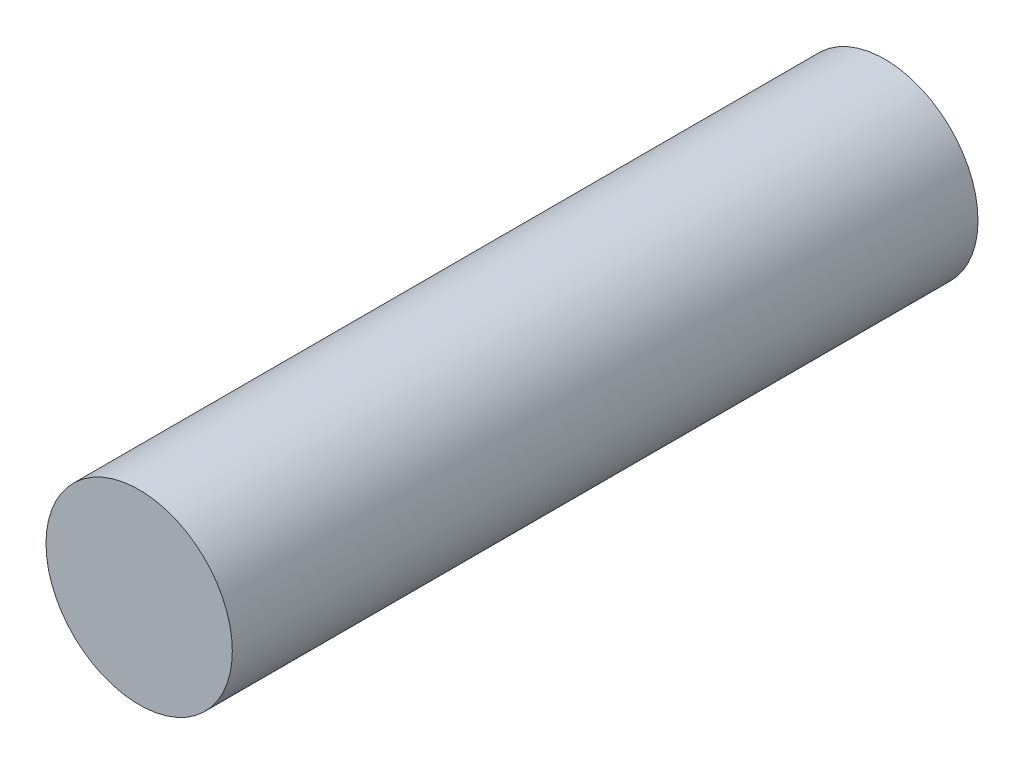
SolidWorks part; units mm, degrees
material "Plain Carbon Steel"
ref_plane "Front Plane" through (0, 0, 0) normal (0, 0, 1) x (1, 0, 0)
ref_plane "Top Plane" through (0, 0, 0) normal (0, 1, 0) x (1, 0, 0)
ref_plane "Right Plane" through (0, 0, 0) normal (1, 0, 0) x (0, 0, -1)
sketch "Pin Profile Ø9.52" plane through (0, 0, 0) normal (0, 0, 1) x (1, 0, 0)
  circle A0 centre (0, 0) radius 4.76
  dimension "D1" = 9.52
extrude "Pin Body L38.1" add sketch "Pin Profile Ø9.52" along normal blind 38.1
